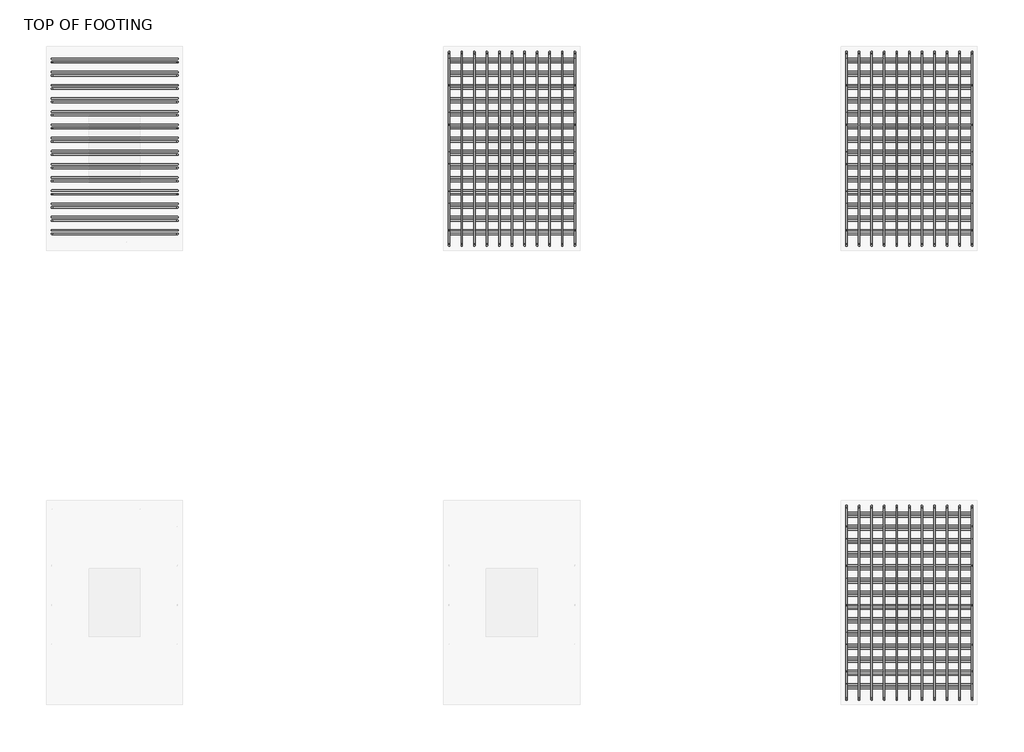
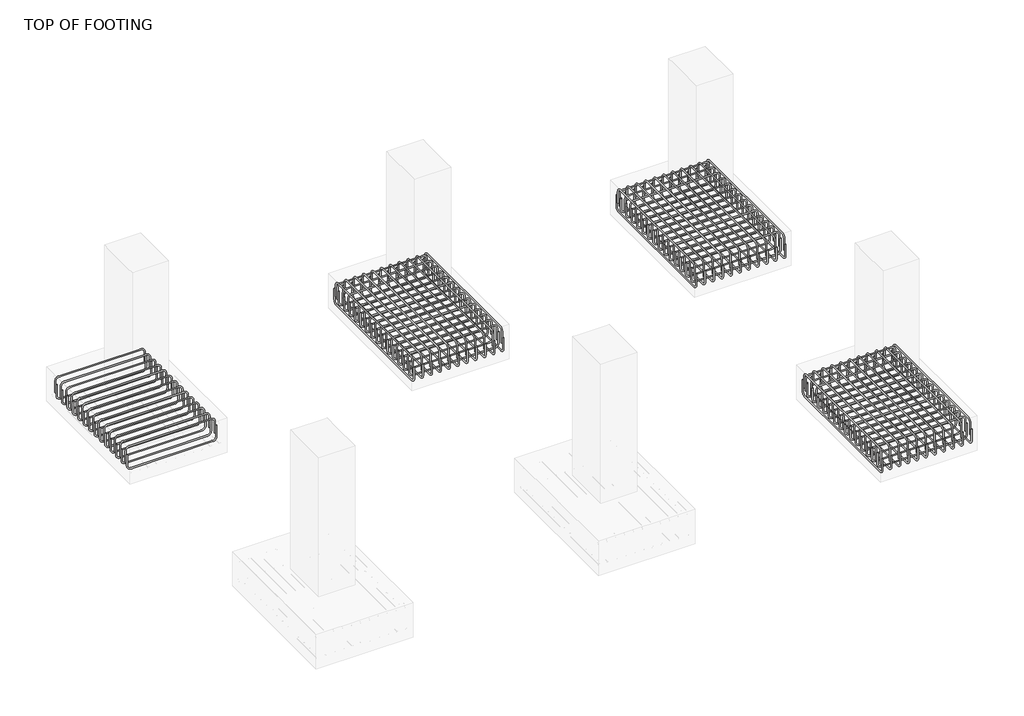
# One storey, part 8 of 11: 14 reinforcing bars.
"""IFC4 building model written with IfcOpenShell, lengths in millimetres."""

from ifc_helpers import new_model, si_unit, point, frame, origin, place, context, project, spatial, polyline, circle_curve, trimmed, segment, composite_curve, source, transform, mapped, element, save
from ifc_brep_helpers import swept_disk

model = new_model("IFC4")

# Units and contexts
model_context = context("Model", 3, world=origin())
ifc_project = project(units=[si_unit("LENGTHUNIT", "METRE", prefix="MILLI")], contexts=[model_context])

# Site, building, storey
site = spatial("IfcSite", under=ifc_project)
building = spatial("IfcBuilding", under=site)
storey = spatial("IfcBuildingStorey", under=building, Name="TOP OF FOOTING", Elevation=-1828.8)

# Reinforcing bars
placement = place(None, origin())
reinforcing_bar_shape = source(origin(), model_context, "Body", "SolidModel", [
    swept_disk(composite_curve([segment(polyline([(8683.7615906, 2549.4712443, -2012.1658531), (8683.7615906, 2549.4712443, -2159.4658531)]), True, "CONTINUOUS"), segment(trimmed(circle_curve(frame((8683.7615906, 2595.8212443, -2159.4658531), z_axis=(1.0, 0.0, 0.0), x_axis=(0.0, -46.350000000000364, 0.0)), 46.35), [point((8683.7615906, 2549.4712443, -2159.4658531))], [point((8683.7615906, 2595.8212443, -2205.8158531))], True, "CARTESIAN"), True, "CONTINUOUS"), segment(polyline([(8683.7615906, 2595.8212443, -2205.8158531), (8683.7615906, 4210.4212443, -2205.8158531)]), True, "CONTINUOUS"), segment(trimmed(circle_curve(frame((8683.7615906, 4210.4212443, -2159.4658531), z_axis=(1.0, 0.0, 0.0), x_axis=(0.0, 0.0, -46.34999999999991)), 46.35), [point((8683.7615906, 4210.4212443, -2205.8158531))], [point((8683.7615906, 4256.7712443, -2159.4658531))], True, "CARTESIAN"), True, "CONTINUOUS"), segment(polyline([(8683.7615906, 4256.7712443, -2159.4658531), (8683.7615906, 4256.7712443, -2012.1658531)]), True, "CONTINUOUS")], self_intersect=False), 6.35),
])
element("IfcReinforcingBar", 1, at=placement, inside=storey, context=model_context, shape_type="MappedRepresentation", body=[
    mapped(reinforcing_bar_shape, transform((0.0, 0.0, 0.0), x_axis=(1.0, 0.0, 0.0), y_axis=(0.0, 1.0, 0.0), z_axis=(0.0, 0.0, 1.0))),
    mapped(reinforcing_bar_shape, transform((-110.73, 0.0, 0.0), x_axis=(1.0, 0.0, 0.0), y_axis=(0.0, 1.0, 0.0), z_axis=(0.0, 0.0, 1.0))),
    mapped(reinforcing_bar_shape, transform((-221.46, 0.0, 0.0), x_axis=(1.0, 0.0, 0.0), y_axis=(0.0, 1.0, 0.0), z_axis=(0.0, 0.0, 1.0))),
    mapped(reinforcing_bar_shape, transform((-332.19, 0.0, 0.0), x_axis=(1.0, 0.0, 0.0), y_axis=(0.0, 1.0, 0.0), z_axis=(0.0, 0.0, 1.0))),
    mapped(reinforcing_bar_shape, transform((-442.92, 0.0, 0.0), x_axis=(1.0, 0.0, 0.0), y_axis=(0.0, 1.0, 0.0), z_axis=(0.0, 0.0, 1.0))),
    mapped(reinforcing_bar_shape, transform((-553.65, 0.0, 0.0), x_axis=(1.0, 0.0, 0.0), y_axis=(0.0, 1.0, 0.0), z_axis=(0.0, 0.0, 1.0))),
    mapped(reinforcing_bar_shape, transform((-664.38, 0.0, 0.0), x_axis=(1.0, 0.0, 0.0), y_axis=(0.0, 1.0, 0.0), z_axis=(0.0, 0.0, 1.0))),
    mapped(reinforcing_bar_shape, transform((-775.11, 0.0, 0.0), x_axis=(1.0, 0.0, 0.0), y_axis=(0.0, 1.0, 0.0), z_axis=(0.0, 0.0, 1.0))),
    mapped(reinforcing_bar_shape, transform((-885.84, 0.0, 0.0), x_axis=(1.0, 0.0, 0.0), y_axis=(0.0, 1.0, 0.0), z_axis=(0.0, 0.0, 1.0))),
    mapped(reinforcing_bar_shape, transform((-996.57, 0.0, 0.0), x_axis=(1.0, 0.0, 0.0), y_axis=(0.0, 1.0, 0.0), z_axis=(0.0, 0.0, 1.0))),
    mapped(reinforcing_bar_shape, transform((-1107.3, 0.0, 0.0), x_axis=(1.0, 0.0, 0.0), y_axis=(0.0, 1.0, 0.0), z_axis=(0.0, 0.0, 1.0))),
])
reinforcing_bar_2_shape = source(origin(), model_context, "Body", "SolidModel", [
    swept_disk(composite_curve([segment(polyline([(7576.4615906, 2577.6603603, -2096.8914539), (7576.4615906, 2577.6603603, -1949.5914539)]), True, "CONTINUOUS"), segment(trimmed(circle_curve(frame((7576.4615906, 2624.0103603, -1949.5914539), z_axis=(-1.0, 0.0, 0.0), x_axis=(0.0, -46.34999999999991, 0.0)), 46.35), [point((7576.4615906, 2577.6603603, -1949.5914539))], [point((7576.4615906, 2624.0103603, -1903.2414539))], True, "CARTESIAN"), True, "CONTINUOUS"), segment(polyline([(7576.4615906, 2624.0103603, -1903.2414539), (7576.4615906, 4181.3238837, -1903.2414539)]), True, "CONTINUOUS"), segment(trimmed(circle_curve(frame((7576.4615906, 4181.3238837, -1949.5914539), z_axis=(-1.0, 0.0, 0.0), x_axis=(0.0, 0.0, 46.350000000000136)), 46.35), [point((7576.4615906, 4181.3238837, -1903.2414539))], [point((7576.4615906, 4227.6738837, -1949.5914539))], True, "CARTESIAN"), True, "CONTINUOUS"), segment(polyline([(7576.4615906, 4227.6738837, -1949.5914539), (7576.4615906, 4227.6738837, -2096.8914539)]), True, "CONTINUOUS")], self_intersect=False), 6.35),
])
element("IfcReinforcingBar", 2, at=placement, inside=storey, context=model_context, shape_type="MappedRepresentation", body=[
    mapped(reinforcing_bar_2_shape, transform((0.0, 0.0, 0.0), x_axis=(1.0, 0.0, 0.0), y_axis=(0.0, 1.0, 0.0), z_axis=(0.0, 0.0, 1.0))),
    mapped(reinforcing_bar_2_shape, transform((110.73, 0.0, 0.0), x_axis=(1.0, 0.0, 0.0), y_axis=(0.0, 1.0, 0.0), z_axis=(0.0, 0.0, 1.0))),
    mapped(reinforcing_bar_2_shape, transform((221.46, 0.0, 0.0), x_axis=(1.0, 0.0, 0.0), y_axis=(0.0, 1.0, 0.0), z_axis=(0.0, 0.0, 1.0))),
    mapped(reinforcing_bar_2_shape, transform((332.19, 0.0, 0.0), x_axis=(1.0, 0.0, 0.0), y_axis=(0.0, 1.0, 0.0), z_axis=(0.0, 0.0, 1.0))),
    mapped(reinforcing_bar_2_shape, transform((442.92, 0.0, 0.0), x_axis=(1.0, 0.0, 0.0), y_axis=(0.0, 1.0, 0.0), z_axis=(0.0, 0.0, 1.0))),
    mapped(reinforcing_bar_2_shape, transform((553.65, 0.0, 0.0), x_axis=(1.0, 0.0, 0.0), y_axis=(0.0, 1.0, 0.0), z_axis=(0.0, 0.0, 1.0))),
    mapped(reinforcing_bar_2_shape, transform((664.38, 0.0, 0.0), x_axis=(1.0, 0.0, 0.0), y_axis=(0.0, 1.0, 0.0), z_axis=(0.0, 0.0, 1.0))),
    mapped(reinforcing_bar_2_shape, transform((775.11, 0.0, 0.0), x_axis=(1.0, 0.0, 0.0), y_axis=(0.0, 1.0, 0.0), z_axis=(0.0, 0.0, 1.0))),
    mapped(reinforcing_bar_2_shape, transform((885.84, 0.0, 0.0), x_axis=(1.0, 0.0, 0.0), y_axis=(0.0, 1.0, 0.0), z_axis=(0.0, 0.0, 1.0))),
    mapped(reinforcing_bar_2_shape, transform((996.57, 0.0, 0.0), x_axis=(1.0, 0.0, 0.0), y_axis=(0.0, 1.0, 0.0), z_axis=(0.0, 0.0, 1.0))),
    mapped(reinforcing_bar_2_shape, transform((1107.3, 0.0, 0.0), x_axis=(1.0, 0.0, 0.0), y_axis=(0.0, 1.0, 0.0), z_axis=(0.0, 0.0, 1.0))),
])
reinforcing_bar_3_shape = source(origin(), model_context, "Body", "SolidModel", [
    swept_disk(composite_curve([segment(polyline([(7576.4615906, 2653.1930221, -1996.7664426), (7576.4615906, 2653.1930221, -2144.0664426)]), True, "CONTINUOUS"), segment(trimmed(circle_curve(frame((7622.8115906, 2653.1930221, -2144.0664426), z_axis=(0.0, -1.0, 0.0), x_axis=(-46.350000000000364, 0.0, 0.0)), 46.35), [point((7576.4615906, 2653.1930221, -2144.0664426))], [point((7622.8115906, 2653.1930221, -2190.4164426))], True, "CARTESIAN"), True, "CONTINUOUS"), segment(polyline([(7622.8115906, 2653.1930221, -2190.4164426), (8637.4115906, 2653.1930221, -2190.4164426)]), True, "CONTINUOUS"), segment(trimmed(circle_curve(frame((8637.4115906, 2653.1930221, -2144.0664426), z_axis=(0.0, -1.0, 0.0), x_axis=(0.0, 0.0, -46.350000000000364)), 46.35), [point((8637.4115906, 2653.1930221, -2190.4164426))], [point((8683.7615906, 2653.1930221, -2144.0664426))], True, "CARTESIAN"), True, "CONTINUOUS"), segment(polyline([(8683.7615906, 2653.1930221, -2144.0664426), (8683.7615906, 2653.1930221, -1996.7664426)]), True, "CONTINUOUS")], self_intersect=False), 6.35),
])
element("IfcReinforcingBar", 3, at=placement, inside=storey, context=model_context, shape_type="MappedRepresentation", body=[
    mapped(reinforcing_bar_3_shape, transform((0.0, 0.0, 0.0), x_axis=(1.0, 0.0, 0.0), y_axis=(0.0, 1.0, 0.0), z_axis=(0.0, 0.0, 1.0))),
    mapped(reinforcing_bar_3_shape, transform((0.0, 116.2744005, 0.0), x_axis=(1.0, 0.0, 0.0), y_axis=(0.0, 1.0, 0.0), z_axis=(0.0, 0.0, 1.0))),
    mapped(reinforcing_bar_3_shape, transform((0.0, 232.5488009, 0.0), x_axis=(1.0, 0.0, 0.0), y_axis=(0.0, 1.0, 0.0), z_axis=(0.0, 0.0, 1.0))),
    mapped(reinforcing_bar_3_shape, transform((0.0, 348.8232014, 0.0), x_axis=(1.0, 0.0, 0.0), y_axis=(0.0, 1.0, 0.0), z_axis=(0.0, 0.0, 1.0))),
    mapped(reinforcing_bar_3_shape, transform((0.0, 465.0976018, 0.0), x_axis=(1.0, 0.0, 0.0), y_axis=(0.0, 1.0, 0.0), z_axis=(0.0, 0.0, 1.0))),
    mapped(reinforcing_bar_3_shape, transform((0.0, 581.3720023, 0.0), x_axis=(1.0, 0.0, 0.0), y_axis=(0.0, 1.0, 0.0), z_axis=(0.0, 0.0, 1.0))),
    mapped(reinforcing_bar_3_shape, transform((0.0, 697.6464027, 0.0), x_axis=(1.0, 0.0, 0.0), y_axis=(0.0, 1.0, 0.0), z_axis=(0.0, 0.0, 1.0))),
    mapped(reinforcing_bar_3_shape, transform((0.0, 813.9208032, 0.0), x_axis=(1.0, 0.0, 0.0), y_axis=(0.0, 1.0, 0.0), z_axis=(0.0, 0.0, 1.0))),
    mapped(reinforcing_bar_3_shape, transform((0.0, 930.1952036, 0.0), x_axis=(1.0, 0.0, 0.0), y_axis=(0.0, 1.0, 0.0), z_axis=(0.0, 0.0, 1.0))),
    mapped(reinforcing_bar_3_shape, transform((0.0, 1046.4696041, 0.0), x_axis=(1.0, 0.0, 0.0), y_axis=(0.0, 1.0, 0.0), z_axis=(0.0, 0.0, 1.0))),
    mapped(reinforcing_bar_3_shape, transform((0.0, 1162.7440045, 0.0), x_axis=(1.0, 0.0, 0.0), y_axis=(0.0, 1.0, 0.0), z_axis=(0.0, 0.0, 1.0))),
    mapped(reinforcing_bar_3_shape, transform((0.0, 1279.018405, 0.0), x_axis=(1.0, 0.0, 0.0), y_axis=(0.0, 1.0, 0.0), z_axis=(0.0, 0.0, 1.0))),
    mapped(reinforcing_bar_3_shape, transform((0.0, 1395.2928054, 0.0), x_axis=(1.0, 0.0, 0.0), y_axis=(0.0, 1.0, 0.0), z_axis=(0.0, 0.0, 1.0))),
    mapped(reinforcing_bar_3_shape, transform((0.0, 1511.5672059, 0.0), x_axis=(1.0, 0.0, 0.0), y_axis=(0.0, 1.0, 0.0), z_axis=(0.0, 0.0, 1.0))),
])
reinforcing_bar_4_shape = source(origin(), model_context, "Body", "SolidModel", [
    swept_disk(composite_curve([segment(polyline([(7576.4615906, 4194.4257435, -2114.1958609), (7576.4615906, 4194.4257435, -1966.8958609)]), True, "CONTINUOUS"), segment(trimmed(circle_curve(frame((7622.8115906, 4194.4257435, -1966.8958609), z_axis=(0.0, 1.0, 0.0), x_axis=(-46.350000000000364, 0.0, 0.0)), 46.35), [point((7576.4615906, 4194.4257435, -1966.8958609))], [point((7622.8115906, 4194.4257435, -1920.5458609))], True, "CARTESIAN"), True, "CONTINUOUS"), segment(polyline([(7622.8115906, 4194.4257435, -1920.5458609), (8637.4115906, 4194.4257435, -1920.5458609)]), True, "CONTINUOUS"), segment(trimmed(circle_curve(frame((8637.4115906, 4194.4257435, -1966.8958609), z_axis=(0.0, 1.0, 0.0), x_axis=(0.0, 0.0, 46.34999999999991)), 46.35), [point((8637.4115906, 4194.4257435, -1920.5458609))], [point((8683.7615906, 4194.4257435, -1966.8958609))], True, "CARTESIAN"), True, "CONTINUOUS"), segment(polyline([(8683.7615906, 4194.4257435, -1966.8958609), (8683.7615906, 4194.4257435, -2114.1958609)]), True, "CONTINUOUS")], self_intersect=False), 6.35),
])
element("IfcReinforcingBar", 4, at=placement, inside=storey, context=model_context, shape_type="MappedRepresentation", body=[
    mapped(reinforcing_bar_4_shape, transform((0.0, 0.0, 0.0), x_axis=(1.0, 0.0, 0.0), y_axis=(0.0, 1.0, 0.0), z_axis=(0.0, 0.0, 1.0))),
    mapped(reinforcing_bar_4_shape, transform((0.0, -116.1057918, 0.0), x_axis=(1.0, 0.0, 0.0), y_axis=(0.0, 1.0, 0.0), z_axis=(0.0, 0.0, 1.0))),
    mapped(reinforcing_bar_4_shape, transform((0.0, -232.2115836, 0.0), x_axis=(1.0, 0.0, 0.0), y_axis=(0.0, 1.0, 0.0), z_axis=(0.0, 0.0, 1.0))),
    mapped(reinforcing_bar_4_shape, transform((0.0, -348.3173754, 0.0), x_axis=(1.0, 0.0, 0.0), y_axis=(0.0, 1.0, 0.0), z_axis=(0.0, 0.0, 1.0))),
    mapped(reinforcing_bar_4_shape, transform((0.0, -464.4231672, 0.0), x_axis=(1.0, 0.0, 0.0), y_axis=(0.0, 1.0, 0.0), z_axis=(0.0, 0.0, 1.0))),
    mapped(reinforcing_bar_4_shape, transform((0.0, -580.528959, 0.0), x_axis=(1.0, 0.0, 0.0), y_axis=(0.0, 1.0, 0.0), z_axis=(0.0, 0.0, 1.0))),
    mapped(reinforcing_bar_4_shape, transform((0.0, -696.6347508, 0.0), x_axis=(1.0, 0.0, 0.0), y_axis=(0.0, 1.0, 0.0), z_axis=(0.0, 0.0, 1.0))),
    mapped(reinforcing_bar_4_shape, transform((0.0, -812.7405426, 0.0), x_axis=(1.0, 0.0, 0.0), y_axis=(0.0, 1.0, 0.0), z_axis=(0.0, 0.0, 1.0))),
    mapped(reinforcing_bar_4_shape, transform((0.0, -928.8463344, 0.0), x_axis=(1.0, 0.0, 0.0), y_axis=(0.0, 1.0, 0.0), z_axis=(0.0, 0.0, 1.0))),
    mapped(reinforcing_bar_4_shape, transform((0.0, -1044.9521262, 0.0), x_axis=(1.0, 0.0, 0.0), y_axis=(0.0, 1.0, 0.0), z_axis=(0.0, 0.0, 1.0))),
    mapped(reinforcing_bar_4_shape, transform((0.0, -1161.057918, 0.0), x_axis=(1.0, 0.0, 0.0), y_axis=(0.0, 1.0, 0.0), z_axis=(0.0, 0.0, 1.0))),
    mapped(reinforcing_bar_4_shape, transform((0.0, -1277.1637098, 0.0), x_axis=(1.0, 0.0, 0.0), y_axis=(0.0, 1.0, 0.0), z_axis=(0.0, 0.0, 1.0))),
    mapped(reinforcing_bar_4_shape, transform((0.0, -1393.2695016, 0.0), x_axis=(1.0, 0.0, 0.0), y_axis=(0.0, 1.0, 0.0), z_axis=(0.0, 0.0, 1.0))),
    mapped(reinforcing_bar_4_shape, transform((0.0, -1509.3752934, 0.0), x_axis=(1.0, 0.0, 0.0), y_axis=(0.0, 1.0, 0.0), z_axis=(0.0, 0.0, 1.0))),
])
reinforcing_bar_5_shape = source(origin(), model_context, "Body", "SolidModel", [
    swept_disk(composite_curve([segment(polyline([(8683.7615906, 6549.4712443, -2012.1658531), (8683.7615906, 6549.4712443, -2159.4658531)]), True, "CONTINUOUS"), segment(trimmed(circle_curve(frame((8683.7615906, 6595.8212443, -2159.4658531), z_axis=(1.0, 0.0, 0.0), x_axis=(0.0, -46.350000000000364, 0.0)), 46.35), [point((8683.7615906, 6549.4712443, -2159.4658531))], [point((8683.7615906, 6595.8212443, -2205.8158531))], True, "CARTESIAN"), True, "CONTINUOUS"), segment(polyline([(8683.7615906, 6595.8212443, -2205.8158531), (8683.7615906, 8210.4212443, -2205.8158531)]), True, "CONTINUOUS"), segment(trimmed(circle_curve(frame((8683.7615906, 8210.4212443, -2159.4658531), z_axis=(1.0, 0.0, 0.0), x_axis=(0.0, 0.0, -46.34999999999991)), 46.35), [point((8683.7615906, 8210.4212443, -2205.8158531))], [point((8683.7615906, 8256.7712443, -2159.4658531))], True, "CARTESIAN"), True, "CONTINUOUS"), segment(polyline([(8683.7615906, 8256.7712443, -2159.4658531), (8683.7615906, 8256.7712443, -2012.1658531)]), True, "CONTINUOUS")], self_intersect=False), 6.35),
])
element("IfcReinforcingBar", 5, at=placement, inside=storey, context=model_context, shape_type="MappedRepresentation", body=[
    mapped(reinforcing_bar_5_shape, transform((0.0, 0.0, 0.0), x_axis=(1.0, 0.0, 0.0), y_axis=(0.0, 1.0, 0.0), z_axis=(0.0, 0.0, 1.0))),
    mapped(reinforcing_bar_5_shape, transform((-110.73, 0.0, 0.0), x_axis=(1.0, 0.0, 0.0), y_axis=(0.0, 1.0, 0.0), z_axis=(0.0, 0.0, 1.0))),
    mapped(reinforcing_bar_5_shape, transform((-221.46, 0.0, 0.0), x_axis=(1.0, 0.0, 0.0), y_axis=(0.0, 1.0, 0.0), z_axis=(0.0, 0.0, 1.0))),
    mapped(reinforcing_bar_5_shape, transform((-332.19, 0.0, 0.0), x_axis=(1.0, 0.0, 0.0), y_axis=(0.0, 1.0, 0.0), z_axis=(0.0, 0.0, 1.0))),
    mapped(reinforcing_bar_5_shape, transform((-442.92, 0.0, 0.0), x_axis=(1.0, 0.0, 0.0), y_axis=(0.0, 1.0, 0.0), z_axis=(0.0, 0.0, 1.0))),
    mapped(reinforcing_bar_5_shape, transform((-553.65, 0.0, 0.0), x_axis=(1.0, 0.0, 0.0), y_axis=(0.0, 1.0, 0.0), z_axis=(0.0, 0.0, 1.0))),
    mapped(reinforcing_bar_5_shape, transform((-664.38, 0.0, 0.0), x_axis=(1.0, 0.0, 0.0), y_axis=(0.0, 1.0, 0.0), z_axis=(0.0, 0.0, 1.0))),
    mapped(reinforcing_bar_5_shape, transform((-775.11, 0.0, 0.0), x_axis=(1.0, 0.0, 0.0), y_axis=(0.0, 1.0, 0.0), z_axis=(0.0, 0.0, 1.0))),
    mapped(reinforcing_bar_5_shape, transform((-885.84, 0.0, 0.0), x_axis=(1.0, 0.0, 0.0), y_axis=(0.0, 1.0, 0.0), z_axis=(0.0, 0.0, 1.0))),
    mapped(reinforcing_bar_5_shape, transform((-996.57, 0.0, 0.0), x_axis=(1.0, 0.0, 0.0), y_axis=(0.0, 1.0, 0.0), z_axis=(0.0, 0.0, 1.0))),
    mapped(reinforcing_bar_5_shape, transform((-1107.3, 0.0, 0.0), x_axis=(1.0, 0.0, 0.0), y_axis=(0.0, 1.0, 0.0), z_axis=(0.0, 0.0, 1.0))),
])
reinforcing_bar_6_shape = source(origin(), model_context, "Body", "SolidModel", [
    swept_disk(composite_curve([segment(polyline([(7576.4615906, 6577.6603603, -2096.8914539), (7576.4615906, 6577.6603603, -1949.5914539)]), True, "CONTINUOUS"), segment(trimmed(circle_curve(frame((7576.4615906, 6624.0103603, -1949.5914539), z_axis=(-1.0, 0.0, 0.0), x_axis=(0.0, -46.349999999999454, 0.0)), 46.35), [point((7576.4615906, 6577.6603603, -1949.5914539))], [point((7576.4615906, 6624.0103603, -1903.2414539))], True, "CARTESIAN"), True, "CONTINUOUS"), segment(polyline([(7576.4615906, 6624.0103603, -1903.2414539), (7576.4615906, 8181.3238837, -1903.2414539)]), True, "CONTINUOUS"), segment(trimmed(circle_curve(frame((7576.4615906, 8181.3238837, -1949.5914539), z_axis=(-1.0, 0.0, 0.0), x_axis=(0.0, 0.0, 46.350000000000136)), 46.35), [point((7576.4615906, 8181.3238837, -1903.2414539))], [point((7576.4615906, 8227.6738837, -1949.5914539))], True, "CARTESIAN"), True, "CONTINUOUS"), segment(polyline([(7576.4615906, 8227.6738837, -1949.5914539), (7576.4615906, 8227.6738837, -2096.8914539)]), True, "CONTINUOUS")], self_intersect=False), 6.35),
])
element("IfcReinforcingBar", 6, at=placement, inside=storey, context=model_context, shape_type="MappedRepresentation", body=[
    mapped(reinforcing_bar_6_shape, transform((0.0, 0.0, 0.0), x_axis=(1.0, 0.0, 0.0), y_axis=(0.0, 1.0, 0.0), z_axis=(0.0, 0.0, 1.0))),
    mapped(reinforcing_bar_6_shape, transform((110.73, 0.0, 0.0), x_axis=(1.0, 0.0, 0.0), y_axis=(0.0, 1.0, 0.0), z_axis=(0.0, 0.0, 1.0))),
    mapped(reinforcing_bar_6_shape, transform((221.46, 0.0, 0.0), x_axis=(1.0, 0.0, 0.0), y_axis=(0.0, 1.0, 0.0), z_axis=(0.0, 0.0, 1.0))),
    mapped(reinforcing_bar_6_shape, transform((332.19, 0.0, 0.0), x_axis=(1.0, 0.0, 0.0), y_axis=(0.0, 1.0, 0.0), z_axis=(0.0, 0.0, 1.0))),
    mapped(reinforcing_bar_6_shape, transform((442.92, 0.0, 0.0), x_axis=(1.0, 0.0, 0.0), y_axis=(0.0, 1.0, 0.0), z_axis=(0.0, 0.0, 1.0))),
    mapped(reinforcing_bar_6_shape, transform((553.65, 0.0, 0.0), x_axis=(1.0, 0.0, 0.0), y_axis=(0.0, 1.0, 0.0), z_axis=(0.0, 0.0, 1.0))),
    mapped(reinforcing_bar_6_shape, transform((664.38, 0.0, 0.0), x_axis=(1.0, 0.0, 0.0), y_axis=(0.0, 1.0, 0.0), z_axis=(0.0, 0.0, 1.0))),
    mapped(reinforcing_bar_6_shape, transform((775.11, 0.0, 0.0), x_axis=(1.0, 0.0, 0.0), y_axis=(0.0, 1.0, 0.0), z_axis=(0.0, 0.0, 1.0))),
    mapped(reinforcing_bar_6_shape, transform((885.84, 0.0, 0.0), x_axis=(1.0, 0.0, 0.0), y_axis=(0.0, 1.0, 0.0), z_axis=(0.0, 0.0, 1.0))),
    mapped(reinforcing_bar_6_shape, transform((996.57, 0.0, 0.0), x_axis=(1.0, 0.0, 0.0), y_axis=(0.0, 1.0, 0.0), z_axis=(0.0, 0.0, 1.0))),
    mapped(reinforcing_bar_6_shape, transform((1107.3, 0.0, 0.0), x_axis=(1.0, 0.0, 0.0), y_axis=(0.0, 1.0, 0.0), z_axis=(0.0, 0.0, 1.0))),
])
reinforcing_bar_7_shape = source(origin(), model_context, "Body", "SolidModel", [
    swept_disk(composite_curve([segment(polyline([(7576.4615906, 6653.1930221, -1996.7664426), (7576.4615906, 6653.1930221, -2144.0664426)]), True, "CONTINUOUS"), segment(trimmed(circle_curve(frame((7622.8115906, 6653.1930221, -2144.0664426), z_axis=(0.0, -1.0, 0.0), x_axis=(-46.350000000000364, 0.0, 0.0)), 46.35), [point((7576.4615906, 6653.1930221, -2144.0664426))], [point((7622.8115906, 6653.1930221, -2190.4164426))], True, "CARTESIAN"), True, "CONTINUOUS"), segment(polyline([(7622.8115906, 6653.1930221, -2190.4164426), (8637.4115906, 6653.1930221, -2190.4164426)]), True, "CONTINUOUS"), segment(trimmed(circle_curve(frame((8637.4115906, 6653.1930221, -2144.0664426), z_axis=(0.0, -1.0, 0.0), x_axis=(0.0, 0.0, -46.350000000000364)), 46.35), [point((8637.4115906, 6653.1930221, -2190.4164426))], [point((8683.7615906, 6653.1930221, -2144.0664426))], True, "CARTESIAN"), True, "CONTINUOUS"), segment(polyline([(8683.7615906, 6653.1930221, -2144.0664426), (8683.7615906, 6653.1930221, -1996.7664426)]), True, "CONTINUOUS")], self_intersect=False), 6.35),
])
element("IfcReinforcingBar", 7, at=placement, inside=storey, context=model_context, shape_type="MappedRepresentation", body=[
    mapped(reinforcing_bar_7_shape, transform((0.0, 0.0, 0.0), x_axis=(1.0, 0.0, 0.0), y_axis=(0.0, 1.0, 0.0), z_axis=(0.0, 0.0, 1.0))),
    mapped(reinforcing_bar_7_shape, transform((0.0, 116.2744005, 0.0), x_axis=(1.0, 0.0, 0.0), y_axis=(0.0, 1.0, 0.0), z_axis=(0.0, 0.0, 1.0))),
    mapped(reinforcing_bar_7_shape, transform((0.0, 232.5488009, 0.0), x_axis=(1.0, 0.0, 0.0), y_axis=(0.0, 1.0, 0.0), z_axis=(0.0, 0.0, 1.0))),
    mapped(reinforcing_bar_7_shape, transform((0.0, 348.8232014, 0.0), x_axis=(1.0, 0.0, 0.0), y_axis=(0.0, 1.0, 0.0), z_axis=(0.0, 0.0, 1.0))),
    mapped(reinforcing_bar_7_shape, transform((0.0, 465.0976018, 0.0), x_axis=(1.0, 0.0, 0.0), y_axis=(0.0, 1.0, 0.0), z_axis=(0.0, 0.0, 1.0))),
    mapped(reinforcing_bar_7_shape, transform((0.0, 581.3720023, 0.0), x_axis=(1.0, 0.0, 0.0), y_axis=(0.0, 1.0, 0.0), z_axis=(0.0, 0.0, 1.0))),
    mapped(reinforcing_bar_7_shape, transform((0.0, 697.6464027, 0.0), x_axis=(1.0, 0.0, 0.0), y_axis=(0.0, 1.0, 0.0), z_axis=(0.0, 0.0, 1.0))),
    mapped(reinforcing_bar_7_shape, transform((0.0, 813.9208032, 0.0), x_axis=(1.0, 0.0, 0.0), y_axis=(0.0, 1.0, 0.0), z_axis=(0.0, 0.0, 1.0))),
    mapped(reinforcing_bar_7_shape, transform((0.0, 930.1952036, 0.0), x_axis=(1.0, 0.0, 0.0), y_axis=(0.0, 1.0, 0.0), z_axis=(0.0, 0.0, 1.0))),
    mapped(reinforcing_bar_7_shape, transform((0.0, 1046.4696041, 0.0), x_axis=(1.0, 0.0, 0.0), y_axis=(0.0, 1.0, 0.0), z_axis=(0.0, 0.0, 1.0))),
    mapped(reinforcing_bar_7_shape, transform((0.0, 1162.7440045, 0.0), x_axis=(1.0, 0.0, 0.0), y_axis=(0.0, 1.0, 0.0), z_axis=(0.0, 0.0, 1.0))),
    mapped(reinforcing_bar_7_shape, transform((0.0, 1279.018405, 0.0), x_axis=(1.0, 0.0, 0.0), y_axis=(0.0, 1.0, 0.0), z_axis=(0.0, 0.0, 1.0))),
    mapped(reinforcing_bar_7_shape, transform((0.0, 1395.2928054, 0.0), x_axis=(1.0, 0.0, 0.0), y_axis=(0.0, 1.0, 0.0), z_axis=(0.0, 0.0, 1.0))),
    mapped(reinforcing_bar_7_shape, transform((0.0, 1511.5672059, 0.0), x_axis=(1.0, 0.0, 0.0), y_axis=(0.0, 1.0, 0.0), z_axis=(0.0, 0.0, 1.0))),
])
reinforcing_bar_8_shape = source(origin(), model_context, "Body", "SolidModel", [
    swept_disk(composite_curve([segment(polyline([(7576.4615906, 8194.4257435, -2114.1958609), (7576.4615906, 8194.4257435, -1966.8958609)]), True, "CONTINUOUS"), segment(trimmed(circle_curve(frame((7622.8115906, 8194.4257435, -1966.8958609), z_axis=(0.0, 1.0, 0.0), x_axis=(-46.350000000000364, 0.0, 0.0)), 46.35), [point((7576.4615906, 8194.4257435, -1966.8958609))], [point((7622.8115906, 8194.4257435, -1920.5458609))], True, "CARTESIAN"), True, "CONTINUOUS"), segment(polyline([(7622.8115906, 8194.4257435, -1920.5458609), (8637.4115906, 8194.4257435, -1920.5458609)]), True, "CONTINUOUS"), segment(trimmed(circle_curve(frame((8637.4115906, 8194.4257435, -1966.8958609), z_axis=(0.0, 1.0, 0.0), x_axis=(0.0, 0.0, 46.34999999999991)), 46.35), [point((8637.4115906, 8194.4257435, -1920.5458609))], [point((8683.7615906, 8194.4257435, -1966.8958609))], True, "CARTESIAN"), True, "CONTINUOUS"), segment(polyline([(8683.7615906, 8194.4257435, -1966.8958609), (8683.7615906, 8194.4257435, -2114.1958609)]), True, "CONTINUOUS")], self_intersect=False), 6.35),
])
element("IfcReinforcingBar", 8, at=placement, inside=storey, context=model_context, shape_type="MappedRepresentation", body=[
    mapped(reinforcing_bar_8_shape, transform((0.0, 0.0, 0.0), x_axis=(1.0, 0.0, 0.0), y_axis=(0.0, 1.0, 0.0), z_axis=(0.0, 0.0, 1.0))),
    mapped(reinforcing_bar_8_shape, transform((0.0, -116.1057918, 0.0), x_axis=(1.0, 0.0, 0.0), y_axis=(0.0, 1.0, 0.0), z_axis=(0.0, 0.0, 1.0))),
    mapped(reinforcing_bar_8_shape, transform((0.0, -232.2115836, 0.0), x_axis=(1.0, 0.0, 0.0), y_axis=(0.0, 1.0, 0.0), z_axis=(0.0, 0.0, 1.0))),
    mapped(reinforcing_bar_8_shape, transform((0.0, -348.3173754, 0.0), x_axis=(1.0, 0.0, 0.0), y_axis=(0.0, 1.0, 0.0), z_axis=(0.0, 0.0, 1.0))),
    mapped(reinforcing_bar_8_shape, transform((0.0, -464.4231672, 0.0), x_axis=(1.0, 0.0, 0.0), y_axis=(0.0, 1.0, 0.0), z_axis=(0.0, 0.0, 1.0))),
    mapped(reinforcing_bar_8_shape, transform((0.0, -580.528959, 0.0), x_axis=(1.0, 0.0, 0.0), y_axis=(0.0, 1.0, 0.0), z_axis=(0.0, 0.0, 1.0))),
    mapped(reinforcing_bar_8_shape, transform((0.0, -696.6347508, 0.0), x_axis=(1.0, 0.0, 0.0), y_axis=(0.0, 1.0, 0.0), z_axis=(0.0, 0.0, 1.0))),
    mapped(reinforcing_bar_8_shape, transform((0.0, -812.7405426, 0.0), x_axis=(1.0, 0.0, 0.0), y_axis=(0.0, 1.0, 0.0), z_axis=(0.0, 0.0, 1.0))),
    mapped(reinforcing_bar_8_shape, transform((0.0, -928.8463344, 0.0), x_axis=(1.0, 0.0, 0.0), y_axis=(0.0, 1.0, 0.0), z_axis=(0.0, 0.0, 1.0))),
    mapped(reinforcing_bar_8_shape, transform((0.0, -1044.9521262, 0.0), x_axis=(1.0, 0.0, 0.0), y_axis=(0.0, 1.0, 0.0), z_axis=(0.0, 0.0, 1.0))),
    mapped(reinforcing_bar_8_shape, transform((0.0, -1161.057918, 0.0), x_axis=(1.0, 0.0, 0.0), y_axis=(0.0, 1.0, 0.0), z_axis=(0.0, 0.0, 1.0))),
    mapped(reinforcing_bar_8_shape, transform((0.0, -1277.1637098, 0.0), x_axis=(1.0, 0.0, 0.0), y_axis=(0.0, 1.0, 0.0), z_axis=(0.0, 0.0, 1.0))),
    mapped(reinforcing_bar_8_shape, transform((0.0, -1393.2695016, 0.0), x_axis=(1.0, 0.0, 0.0), y_axis=(0.0, 1.0, 0.0), z_axis=(0.0, 0.0, 1.0))),
    mapped(reinforcing_bar_8_shape, transform((0.0, -1509.3752934, 0.0), x_axis=(1.0, 0.0, 0.0), y_axis=(0.0, 1.0, 0.0), z_axis=(0.0, 0.0, 1.0))),
])
reinforcing_bar_9_shape = source(origin(), model_context, "Body", "SolidModel", [
    swept_disk(composite_curve([segment(polyline([(5183.7615906, 6549.4712443, -2012.1658531), (5183.7615906, 6549.4712443, -2159.4658531)]), True, "CONTINUOUS"), segment(trimmed(circle_curve(frame((5183.7615906, 6595.8212443, -2159.4658531), z_axis=(1.0, 0.0, 0.0), x_axis=(0.0, -46.350000000000364, 0.0)), 46.35), [point((5183.7615906, 6549.4712443, -2159.4658531))], [point((5183.7615906, 6595.8212443, -2205.8158531))], True, "CARTESIAN"), True, "CONTINUOUS"), segment(polyline([(5183.7615906, 6595.8212443, -2205.8158531), (5183.7615906, 8210.4212443, -2205.8158531)]), True, "CONTINUOUS"), segment(trimmed(circle_curve(frame((5183.7615906, 8210.4212443, -2159.4658531), z_axis=(1.0, 0.0, 0.0), x_axis=(0.0, 0.0, -46.34999999999991)), 46.35), [point((5183.7615906, 8210.4212443, -2205.8158531))], [point((5183.7615906, 8256.7712443, -2159.4658531))], True, "CARTESIAN"), True, "CONTINUOUS"), segment(polyline([(5183.7615906, 8256.7712443, -2159.4658531), (5183.7615906, 8256.7712443, -2012.1658531)]), True, "CONTINUOUS")], self_intersect=False), 6.35),
])
element("IfcReinforcingBar", 9, at=placement, inside=storey, context=model_context, shape_type="MappedRepresentation", body=[
    mapped(reinforcing_bar_9_shape, transform((0.0, 0.0, 0.0), x_axis=(1.0, 0.0, 0.0), y_axis=(0.0, 1.0, 0.0), z_axis=(0.0, 0.0, 1.0))),
    mapped(reinforcing_bar_9_shape, transform((-110.73, 0.0, 0.0), x_axis=(1.0, 0.0, 0.0), y_axis=(0.0, 1.0, 0.0), z_axis=(0.0, 0.0, 1.0))),
    mapped(reinforcing_bar_9_shape, transform((-221.46, 0.0, 0.0), x_axis=(1.0, 0.0, 0.0), y_axis=(0.0, 1.0, 0.0), z_axis=(0.0, 0.0, 1.0))),
    mapped(reinforcing_bar_9_shape, transform((-332.19, 0.0, 0.0), x_axis=(1.0, 0.0, 0.0), y_axis=(0.0, 1.0, 0.0), z_axis=(0.0, 0.0, 1.0))),
    mapped(reinforcing_bar_9_shape, transform((-442.92, 0.0, 0.0), x_axis=(1.0, 0.0, 0.0), y_axis=(0.0, 1.0, 0.0), z_axis=(0.0, 0.0, 1.0))),
    mapped(reinforcing_bar_9_shape, transform((-553.65, 0.0, 0.0), x_axis=(1.0, 0.0, 0.0), y_axis=(0.0, 1.0, 0.0), z_axis=(0.0, 0.0, 1.0))),
    mapped(reinforcing_bar_9_shape, transform((-664.38, 0.0, 0.0), x_axis=(1.0, 0.0, 0.0), y_axis=(0.0, 1.0, 0.0), z_axis=(0.0, 0.0, 1.0))),
    mapped(reinforcing_bar_9_shape, transform((-775.11, 0.0, 0.0), x_axis=(1.0, 0.0, 0.0), y_axis=(0.0, 1.0, 0.0), z_axis=(0.0, 0.0, 1.0))),
    mapped(reinforcing_bar_9_shape, transform((-885.84, 0.0, 0.0), x_axis=(1.0, 0.0, 0.0), y_axis=(0.0, 1.0, 0.0), z_axis=(0.0, 0.0, 1.0))),
    mapped(reinforcing_bar_9_shape, transform((-996.57, 0.0, 0.0), x_axis=(1.0, 0.0, 0.0), y_axis=(0.0, 1.0, 0.0), z_axis=(0.0, 0.0, 1.0))),
    mapped(reinforcing_bar_9_shape, transform((-1107.3, 0.0, 0.0), x_axis=(1.0, 0.0, 0.0), y_axis=(0.0, 1.0, 0.0), z_axis=(0.0, 0.0, 1.0))),
])
reinforcing_bar_10_shape = source(origin(), model_context, "Body", "SolidModel", [
    swept_disk(composite_curve([segment(polyline([(4076.4615906, 6577.6603603, -2096.8914539), (4076.4615906, 6577.6603603, -1949.5914539)]), True, "CONTINUOUS"), segment(trimmed(circle_curve(frame((4076.4615906, 6624.0103603, -1949.5914539), z_axis=(-1.0, 0.0, 0.0), x_axis=(0.0, -46.349999999999454, 0.0)), 46.35), [point((4076.4615906, 6577.6603603, -1949.5914539))], [point((4076.4615906, 6624.0103603, -1903.2414539))], True, "CARTESIAN"), True, "CONTINUOUS"), segment(polyline([(4076.4615906, 6624.0103603, -1903.2414539), (4076.4615906, 8181.3238837, -1903.2414539)]), True, "CONTINUOUS"), segment(trimmed(circle_curve(frame((4076.4615906, 8181.3238837, -1949.5914539), z_axis=(-1.0, 0.0, 0.0), x_axis=(0.0, 0.0, 46.350000000000136)), 46.35), [point((4076.4615906, 8181.3238837, -1903.2414539))], [point((4076.4615906, 8227.6738837, -1949.5914539))], True, "CARTESIAN"), True, "CONTINUOUS"), segment(polyline([(4076.4615906, 8227.6738837, -1949.5914539), (4076.4615906, 8227.6738837, -2096.8914539)]), True, "CONTINUOUS")], self_intersect=False), 6.35),
])
element("IfcReinforcingBar", 10, at=placement, inside=storey, context=model_context, shape_type="MappedRepresentation", body=[
    mapped(reinforcing_bar_10_shape, transform((0.0, 0.0, 0.0), x_axis=(1.0, 0.0, 0.0), y_axis=(0.0, 1.0, 0.0), z_axis=(0.0, 0.0, 1.0))),
    mapped(reinforcing_bar_10_shape, transform((110.73, 0.0, 0.0), x_axis=(1.0, 0.0, 0.0), y_axis=(0.0, 1.0, 0.0), z_axis=(0.0, 0.0, 1.0))),
    mapped(reinforcing_bar_10_shape, transform((221.46, 0.0, 0.0), x_axis=(1.0, 0.0, 0.0), y_axis=(0.0, 1.0, 0.0), z_axis=(0.0, 0.0, 1.0))),
    mapped(reinforcing_bar_10_shape, transform((332.19, 0.0, 0.0), x_axis=(1.0, 0.0, 0.0), y_axis=(0.0, 1.0, 0.0), z_axis=(0.0, 0.0, 1.0))),
    mapped(reinforcing_bar_10_shape, transform((442.92, 0.0, 0.0), x_axis=(1.0, 0.0, 0.0), y_axis=(0.0, 1.0, 0.0), z_axis=(0.0, 0.0, 1.0))),
    mapped(reinforcing_bar_10_shape, transform((553.65, 0.0, 0.0), x_axis=(1.0, 0.0, 0.0), y_axis=(0.0, 1.0, 0.0), z_axis=(0.0, 0.0, 1.0))),
    mapped(reinforcing_bar_10_shape, transform((664.38, 0.0, 0.0), x_axis=(1.0, 0.0, 0.0), y_axis=(0.0, 1.0, 0.0), z_axis=(0.0, 0.0, 1.0))),
    mapped(reinforcing_bar_10_shape, transform((775.11, 0.0, 0.0), x_axis=(1.0, 0.0, 0.0), y_axis=(0.0, 1.0, 0.0), z_axis=(0.0, 0.0, 1.0))),
    mapped(reinforcing_bar_10_shape, transform((885.84, 0.0, 0.0), x_axis=(1.0, 0.0, 0.0), y_axis=(0.0, 1.0, 0.0), z_axis=(0.0, 0.0, 1.0))),
    mapped(reinforcing_bar_10_shape, transform((996.57, 0.0, 0.0), x_axis=(1.0, 0.0, 0.0), y_axis=(0.0, 1.0, 0.0), z_axis=(0.0, 0.0, 1.0))),
    mapped(reinforcing_bar_10_shape, transform((1107.3, 0.0, 0.0), x_axis=(1.0, 0.0, 0.0), y_axis=(0.0, 1.0, 0.0), z_axis=(0.0, 0.0, 1.0))),
])
reinforcing_bar_11_shape = source(origin(), model_context, "Body", "SolidModel", [
    swept_disk(composite_curve([segment(polyline([(4076.4615906, 6653.1930221, -1996.7664426), (4076.4615906, 6653.1930221, -2144.0664426)]), True, "CONTINUOUS"), segment(trimmed(circle_curve(frame((4122.8115906, 6653.1930221, -2144.0664426), z_axis=(0.0, -1.0, 0.0), x_axis=(-46.350000000000364, 0.0, 0.0)), 46.35), [point((4076.4615906, 6653.1930221, -2144.0664426))], [point((4122.8115906, 6653.1930221, -2190.4164426))], True, "CARTESIAN"), True, "CONTINUOUS"), segment(polyline([(4122.8115906, 6653.1930221, -2190.4164426), (5137.4115906, 6653.1930221, -2190.4164426)]), True, "CONTINUOUS"), segment(trimmed(circle_curve(frame((5137.4115906, 6653.1930221, -2144.0664426), z_axis=(0.0, -1.0, 0.0), x_axis=(0.0, 0.0, -46.350000000000364)), 46.35), [point((5137.4115906, 6653.1930221, -2190.4164426))], [point((5183.7615906, 6653.1930221, -2144.0664426))], True, "CARTESIAN"), True, "CONTINUOUS"), segment(polyline([(5183.7615906, 6653.1930221, -2144.0664426), (5183.7615906, 6653.1930221, -1996.7664426)]), True, "CONTINUOUS")], self_intersect=False), 6.35),
])
element("IfcReinforcingBar", 11, at=placement, inside=storey, context=model_context, shape_type="MappedRepresentation", body=[
    mapped(reinforcing_bar_11_shape, transform((0.0, 0.0, 0.0), x_axis=(1.0, 0.0, 0.0), y_axis=(0.0, 1.0, 0.0), z_axis=(0.0, 0.0, 1.0))),
    mapped(reinforcing_bar_11_shape, transform((0.0, 116.2744005, 0.0), x_axis=(1.0, 0.0, 0.0), y_axis=(0.0, 1.0, 0.0), z_axis=(0.0, 0.0, 1.0))),
    mapped(reinforcing_bar_11_shape, transform((0.0, 232.5488009, 0.0), x_axis=(1.0, 0.0, 0.0), y_axis=(0.0, 1.0, 0.0), z_axis=(0.0, 0.0, 1.0))),
    mapped(reinforcing_bar_11_shape, transform((0.0, 348.8232014, 0.0), x_axis=(1.0, 0.0, 0.0), y_axis=(0.0, 1.0, 0.0), z_axis=(0.0, 0.0, 1.0))),
    mapped(reinforcing_bar_11_shape, transform((0.0, 465.0976018, 0.0), x_axis=(1.0, 0.0, 0.0), y_axis=(0.0, 1.0, 0.0), z_axis=(0.0, 0.0, 1.0))),
    mapped(reinforcing_bar_11_shape, transform((0.0, 581.3720023, 0.0), x_axis=(1.0, 0.0, 0.0), y_axis=(0.0, 1.0, 0.0), z_axis=(0.0, 0.0, 1.0))),
    mapped(reinforcing_bar_11_shape, transform((0.0, 697.6464027, 0.0), x_axis=(1.0, 0.0, 0.0), y_axis=(0.0, 1.0, 0.0), z_axis=(0.0, 0.0, 1.0))),
    mapped(reinforcing_bar_11_shape, transform((0.0, 813.9208032, 0.0), x_axis=(1.0, 0.0, 0.0), y_axis=(0.0, 1.0, 0.0), z_axis=(0.0, 0.0, 1.0))),
    mapped(reinforcing_bar_11_shape, transform((0.0, 930.1952036, 0.0), x_axis=(1.0, 0.0, 0.0), y_axis=(0.0, 1.0, 0.0), z_axis=(0.0, 0.0, 1.0))),
    mapped(reinforcing_bar_11_shape, transform((0.0, 1046.4696041, 0.0), x_axis=(1.0, 0.0, 0.0), y_axis=(0.0, 1.0, 0.0), z_axis=(0.0, 0.0, 1.0))),
    mapped(reinforcing_bar_11_shape, transform((0.0, 1162.7440045, 0.0), x_axis=(1.0, 0.0, 0.0), y_axis=(0.0, 1.0, 0.0), z_axis=(0.0, 0.0, 1.0))),
    mapped(reinforcing_bar_11_shape, transform((0.0, 1279.018405, 0.0), x_axis=(1.0, 0.0, 0.0), y_axis=(0.0, 1.0, 0.0), z_axis=(0.0, 0.0, 1.0))),
    mapped(reinforcing_bar_11_shape, transform((0.0, 1395.2928054, 0.0), x_axis=(1.0, 0.0, 0.0), y_axis=(0.0, 1.0, 0.0), z_axis=(0.0, 0.0, 1.0))),
    mapped(reinforcing_bar_11_shape, transform((0.0, 1511.5672059, 0.0), x_axis=(1.0, 0.0, 0.0), y_axis=(0.0, 1.0, 0.0), z_axis=(0.0, 0.0, 1.0))),
])
reinforcing_bar_12_shape = source(origin(), model_context, "Body", "SolidModel", [
    swept_disk(composite_curve([segment(polyline([(4076.4615906, 8194.4257435, -2114.1958609), (4076.4615906, 8194.4257435, -1966.8958609)]), True, "CONTINUOUS"), segment(trimmed(circle_curve(frame((4122.8115906, 8194.4257435, -1966.8958609), z_axis=(0.0, 1.0, 0.0), x_axis=(-46.350000000000364, 0.0, 0.0)), 46.35), [point((4076.4615906, 8194.4257435, -1966.8958609))], [point((4122.8115906, 8194.4257435, -1920.5458609))], True, "CARTESIAN"), True, "CONTINUOUS"), segment(polyline([(4122.8115906, 8194.4257435, -1920.5458609), (5137.4115906, 8194.4257435, -1920.5458609)]), True, "CONTINUOUS"), segment(trimmed(circle_curve(frame((5137.4115906, 8194.4257435, -1966.8958609), z_axis=(0.0, 1.0, 0.0), x_axis=(0.0, 0.0, 46.34999999999991)), 46.35), [point((5137.4115906, 8194.4257435, -1920.5458609))], [point((5183.7615906, 8194.4257435, -1966.8958609))], True, "CARTESIAN"), True, "CONTINUOUS"), segment(polyline([(5183.7615906, 8194.4257435, -1966.8958609), (5183.7615906, 8194.4257435, -2114.1958609)]), True, "CONTINUOUS")], self_intersect=False), 6.35),
])
element("IfcReinforcingBar", 12, at=placement, inside=storey, context=model_context, shape_type="MappedRepresentation", body=[
    mapped(reinforcing_bar_12_shape, transform((0.0, 0.0, 0.0), x_axis=(1.0, 0.0, 0.0), y_axis=(0.0, 1.0, 0.0), z_axis=(0.0, 0.0, 1.0))),
    mapped(reinforcing_bar_12_shape, transform((0.0, -116.1057918, 0.0), x_axis=(1.0, 0.0, 0.0), y_axis=(0.0, 1.0, 0.0), z_axis=(0.0, 0.0, 1.0))),
    mapped(reinforcing_bar_12_shape, transform((0.0, -232.2115836, 0.0), x_axis=(1.0, 0.0, 0.0), y_axis=(0.0, 1.0, 0.0), z_axis=(0.0, 0.0, 1.0))),
    mapped(reinforcing_bar_12_shape, transform((0.0, -348.3173754, 0.0), x_axis=(1.0, 0.0, 0.0), y_axis=(0.0, 1.0, 0.0), z_axis=(0.0, 0.0, 1.0))),
    mapped(reinforcing_bar_12_shape, transform((0.0, -464.4231672, 0.0), x_axis=(1.0, 0.0, 0.0), y_axis=(0.0, 1.0, 0.0), z_axis=(0.0, 0.0, 1.0))),
    mapped(reinforcing_bar_12_shape, transform((0.0, -580.528959, 0.0), x_axis=(1.0, 0.0, 0.0), y_axis=(0.0, 1.0, 0.0), z_axis=(0.0, 0.0, 1.0))),
    mapped(reinforcing_bar_12_shape, transform((0.0, -696.6347508, 0.0), x_axis=(1.0, 0.0, 0.0), y_axis=(0.0, 1.0, 0.0), z_axis=(0.0, 0.0, 1.0))),
    mapped(reinforcing_bar_12_shape, transform((0.0, -812.7405426, 0.0), x_axis=(1.0, 0.0, 0.0), y_axis=(0.0, 1.0, 0.0), z_axis=(0.0, 0.0, 1.0))),
    mapped(reinforcing_bar_12_shape, transform((0.0, -928.8463344, 0.0), x_axis=(1.0, 0.0, 0.0), y_axis=(0.0, 1.0, 0.0), z_axis=(0.0, 0.0, 1.0))),
    mapped(reinforcing_bar_12_shape, transform((0.0, -1044.9521262, 0.0), x_axis=(1.0, 0.0, 0.0), y_axis=(0.0, 1.0, 0.0), z_axis=(0.0, 0.0, 1.0))),
    mapped(reinforcing_bar_12_shape, transform((0.0, -1161.057918, 0.0), x_axis=(1.0, 0.0, 0.0), y_axis=(0.0, 1.0, 0.0), z_axis=(0.0, 0.0, 1.0))),
    mapped(reinforcing_bar_12_shape, transform((0.0, -1277.1637098, 0.0), x_axis=(1.0, 0.0, 0.0), y_axis=(0.0, 1.0, 0.0), z_axis=(0.0, 0.0, 1.0))),
    mapped(reinforcing_bar_12_shape, transform((0.0, -1393.2695016, 0.0), x_axis=(1.0, 0.0, 0.0), y_axis=(0.0, 1.0, 0.0), z_axis=(0.0, 0.0, 1.0))),
    mapped(reinforcing_bar_12_shape, transform((0.0, -1509.3752934, 0.0), x_axis=(1.0, 0.0, 0.0), y_axis=(0.0, 1.0, 0.0), z_axis=(0.0, 0.0, 1.0))),
])
reinforcing_bar_13_shape = source(origin(), model_context, "Body", "SolidModel", [
    swept_disk(composite_curve([segment(polyline([(576.4615906, 6653.1930221, -1996.7664426), (576.4615906, 6653.1930221, -2144.0664426)]), True, "CONTINUOUS"), segment(trimmed(circle_curve(frame((622.8115906, 6653.1930221, -2144.0664426), z_axis=(0.0, -1.0, 0.0), x_axis=(-46.35000000000002, 0.0, 0.0)), 46.35), [point((576.4615906, 6653.1930221, -2144.0664426))], [point((622.8115906, 6653.1930221, -2190.4164426))], True, "CARTESIAN"), True, "CONTINUOUS"), segment(polyline([(622.8115906, 6653.1930221, -2190.4164426), (1637.4115906, 6653.1930221, -2190.4164426)]), True, "CONTINUOUS"), segment(trimmed(circle_curve(frame((1637.4115906, 6653.1930221, -2144.0664426), z_axis=(0.0, -1.0, 0.0), x_axis=(0.0, 0.0, -46.350000000000364)), 46.35), [point((1637.4115906, 6653.1930221, -2190.4164426))], [point((1683.7615906, 6653.1930221, -2144.0664426))], True, "CARTESIAN"), True, "CONTINUOUS"), segment(polyline([(1683.7615906, 6653.1930221, -2144.0664426), (1683.7615906, 6653.1930221, -1996.7664426)]), True, "CONTINUOUS")], self_intersect=False), 6.35),
])
element("IfcReinforcingBar", 13, at=placement, inside=storey, context=model_context, shape_type="MappedRepresentation", body=[
    mapped(reinforcing_bar_13_shape, transform((0.0, 0.0, 0.0), x_axis=(1.0, 0.0, 0.0), y_axis=(0.0, 1.0, 0.0), z_axis=(0.0, 0.0, 1.0))),
    mapped(reinforcing_bar_13_shape, transform((0.0, 116.2744005, 0.0), x_axis=(1.0, 0.0, 0.0), y_axis=(0.0, 1.0, 0.0), z_axis=(0.0, 0.0, 1.0))),
    mapped(reinforcing_bar_13_shape, transform((0.0, 232.5488009, 0.0), x_axis=(1.0, 0.0, 0.0), y_axis=(0.0, 1.0, 0.0), z_axis=(0.0, 0.0, 1.0))),
    mapped(reinforcing_bar_13_shape, transform((0.0, 348.8232014, 0.0), x_axis=(1.0, 0.0, 0.0), y_axis=(0.0, 1.0, 0.0), z_axis=(0.0, 0.0, 1.0))),
    mapped(reinforcing_bar_13_shape, transform((0.0, 465.0976018, 0.0), x_axis=(1.0, 0.0, 0.0), y_axis=(0.0, 1.0, 0.0), z_axis=(0.0, 0.0, 1.0))),
    mapped(reinforcing_bar_13_shape, transform((0.0, 581.3720023, 0.0), x_axis=(1.0, 0.0, 0.0), y_axis=(0.0, 1.0, 0.0), z_axis=(0.0, 0.0, 1.0))),
    mapped(reinforcing_bar_13_shape, transform((0.0, 697.6464027, 0.0), x_axis=(1.0, 0.0, 0.0), y_axis=(0.0, 1.0, 0.0), z_axis=(0.0, 0.0, 1.0))),
    mapped(reinforcing_bar_13_shape, transform((0.0, 813.9208032, 0.0), x_axis=(1.0, 0.0, 0.0), y_axis=(0.0, 1.0, 0.0), z_axis=(0.0, 0.0, 1.0))),
    mapped(reinforcing_bar_13_shape, transform((0.0, 930.1952036, 0.0), x_axis=(1.0, 0.0, 0.0), y_axis=(0.0, 1.0, 0.0), z_axis=(0.0, 0.0, 1.0))),
    mapped(reinforcing_bar_13_shape, transform((0.0, 1046.4696041, 0.0), x_axis=(1.0, 0.0, 0.0), y_axis=(0.0, 1.0, 0.0), z_axis=(0.0, 0.0, 1.0))),
    mapped(reinforcing_bar_13_shape, transform((0.0, 1162.7440045, 0.0), x_axis=(1.0, 0.0, 0.0), y_axis=(0.0, 1.0, 0.0), z_axis=(0.0, 0.0, 1.0))),
    mapped(reinforcing_bar_13_shape, transform((0.0, 1279.018405, 0.0), x_axis=(1.0, 0.0, 0.0), y_axis=(0.0, 1.0, 0.0), z_axis=(0.0, 0.0, 1.0))),
    mapped(reinforcing_bar_13_shape, transform((0.0, 1395.2928054, 0.0), x_axis=(1.0, 0.0, 0.0), y_axis=(0.0, 1.0, 0.0), z_axis=(0.0, 0.0, 1.0))),
    mapped(reinforcing_bar_13_shape, transform((0.0, 1511.5672059, 0.0), x_axis=(1.0, 0.0, 0.0), y_axis=(0.0, 1.0, 0.0), z_axis=(0.0, 0.0, 1.0))),
])
reinforcing_bar_14_shape = source(origin(), model_context, "Body", "SolidModel", [
    swept_disk(composite_curve([segment(polyline([(576.4615906, 8194.4257435, -2114.1958609), (576.4615906, 8194.4257435, -1966.8958609)]), True, "CONTINUOUS"), segment(trimmed(circle_curve(frame((622.8115906, 8194.4257435, -1966.8958609), z_axis=(0.0, 1.0, 0.0), x_axis=(-46.35000000000002, 0.0, 0.0)), 46.35), [point((576.4615906, 8194.4257435, -1966.8958609))], [point((622.8115906, 8194.4257435, -1920.5458609))], True, "CARTESIAN"), True, "CONTINUOUS"), segment(polyline([(622.8115906, 8194.4257435, -1920.5458609), (1637.4115906, 8194.4257435, -1920.5458609)]), True, "CONTINUOUS"), segment(trimmed(circle_curve(frame((1637.4115906, 8194.4257435, -1966.8958609), z_axis=(0.0, 1.0, 0.0), x_axis=(0.0, 0.0, 46.34999999999991)), 46.35), [point((1637.4115906, 8194.4257435, -1920.5458609))], [point((1683.7615906, 8194.4257435, -1966.8958609))], True, "CARTESIAN"), True, "CONTINUOUS"), segment(polyline([(1683.7615906, 8194.4257435, -1966.8958609), (1683.7615906, 8194.4257435, -2114.1958609)]), True, "CONTINUOUS")], self_intersect=False), 6.35),
])
element("IfcReinforcingBar", 14, at=placement, inside=storey, context=model_context, shape_type="MappedRepresentation", body=[
    mapped(reinforcing_bar_14_shape, transform((0.0, 0.0, 0.0), x_axis=(1.0, 0.0, 0.0), y_axis=(0.0, 1.0, 0.0), z_axis=(0.0, 0.0, 1.0))),
    mapped(reinforcing_bar_14_shape, transform((0.0, -116.1057918, 0.0), x_axis=(1.0, 0.0, 0.0), y_axis=(0.0, 1.0, 0.0), z_axis=(0.0, 0.0, 1.0))),
    mapped(reinforcing_bar_14_shape, transform((0.0, -232.2115836, 0.0), x_axis=(1.0, 0.0, 0.0), y_axis=(0.0, 1.0, 0.0), z_axis=(0.0, 0.0, 1.0))),
    mapped(reinforcing_bar_14_shape, transform((0.0, -348.3173754, 0.0), x_axis=(1.0, 0.0, 0.0), y_axis=(0.0, 1.0, 0.0), z_axis=(0.0, 0.0, 1.0))),
    mapped(reinforcing_bar_14_shape, transform((0.0, -464.4231672, 0.0), x_axis=(1.0, 0.0, 0.0), y_axis=(0.0, 1.0, 0.0), z_axis=(0.0, 0.0, 1.0))),
    mapped(reinforcing_bar_14_shape, transform((0.0, -580.528959, 0.0), x_axis=(1.0, 0.0, 0.0), y_axis=(0.0, 1.0, 0.0), z_axis=(0.0, 0.0, 1.0))),
    mapped(reinforcing_bar_14_shape, transform((0.0, -696.6347508, 0.0), x_axis=(1.0, 0.0, 0.0), y_axis=(0.0, 1.0, 0.0), z_axis=(0.0, 0.0, 1.0))),
    mapped(reinforcing_bar_14_shape, transform((0.0, -812.7405426, 0.0), x_axis=(1.0, 0.0, 0.0), y_axis=(0.0, 1.0, 0.0), z_axis=(0.0, 0.0, 1.0))),
    mapped(reinforcing_bar_14_shape, transform((0.0, -928.8463344, 0.0), x_axis=(1.0, 0.0, 0.0), y_axis=(0.0, 1.0, 0.0), z_axis=(0.0, 0.0, 1.0))),
    mapped(reinforcing_bar_14_shape, transform((0.0, -1044.9521262, 0.0), x_axis=(1.0, 0.0, 0.0), y_axis=(0.0, 1.0, 0.0), z_axis=(0.0, 0.0, 1.0))),
    mapped(reinforcing_bar_14_shape, transform((0.0, -1161.057918, 0.0), x_axis=(1.0, 0.0, 0.0), y_axis=(0.0, 1.0, 0.0), z_axis=(0.0, 0.0, 1.0))),
    mapped(reinforcing_bar_14_shape, transform((0.0, -1277.1637098, 0.0), x_axis=(1.0, 0.0, 0.0), y_axis=(0.0, 1.0, 0.0), z_axis=(0.0, 0.0, 1.0))),
    mapped(reinforcing_bar_14_shape, transform((0.0, -1393.2695016, 0.0), x_axis=(1.0, 0.0, 0.0), y_axis=(0.0, 1.0, 0.0), z_axis=(0.0, 0.0, 1.0))),
    mapped(reinforcing_bar_14_shape, transform((0.0, -1509.3752934, 0.0), x_axis=(1.0, 0.0, 0.0), y_axis=(0.0, 1.0, 0.0), z_axis=(0.0, 0.0, 1.0))),
])

save(model, "model.ifc")

# Revit data of these elements
# Elements 1, 2, 3, 4, 5, 6, 7, 8, 9, 10, 11, 12, 13, 14 (IfcReinforcingBar)
#   Phase Created = New Construction
